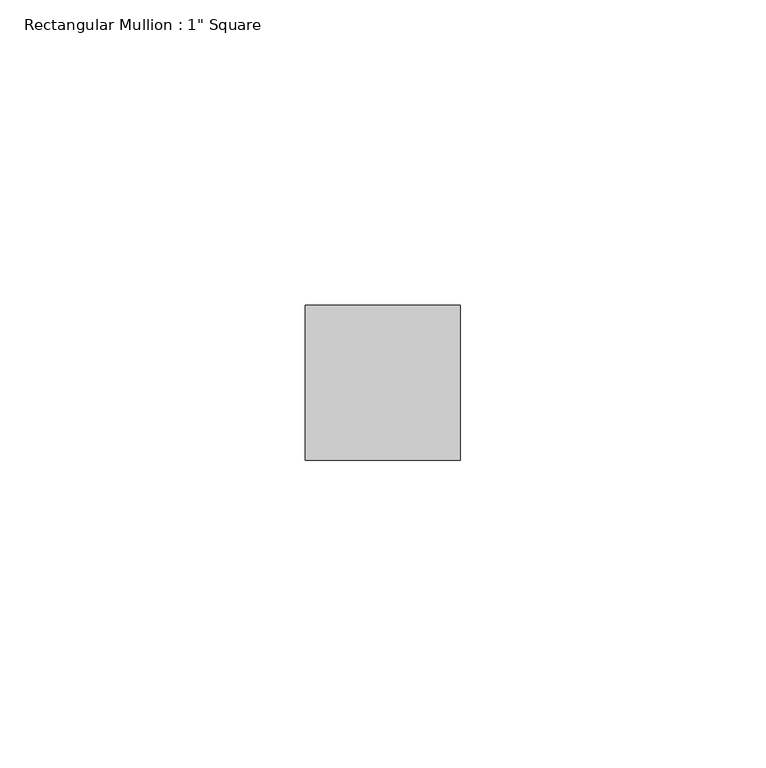
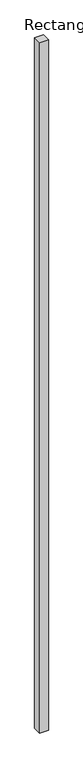
"""IFC4 building model written with IfcOpenShell, lengths in millimetres: member geometry."""

from ifc_helpers import new_model, si_unit, frame, origin, place, context, project, spatial, polyline, outline, extrude, source, transform, mapped, element, save


def member_c125f493(model_context):
    return source(origin(), model_context, "Body", "SweptSolid", [
        extrude(outline(polyline([(12.7, 12.7), (12.7, -12.7), (-12.7, -12.7), (-12.7, 12.7), (12.7, 12.7)])), frame((0.0, 0.0, -2139.95), z_axis=(0.0, 0.0, 1.0), x_axis=(1.0, 0.0, 0.0)), (0.0, 0.0, 1.0), 2139.95),
    ])


if __name__ == "__main__":
    model = new_model("IFC4")
    model_context = context("Model", 3, world=origin())
    ifc_project = project(units=[si_unit("LENGTHUNIT", "METRE", prefix="MILLI")], contexts=[model_context])
    site = spatial("IfcSite", under=ifc_project)
    building = spatial("IfcBuilding", under=site)
    placement = place(None, origin())
    member_shape = member_c125f493(model_context)
    element("IfcMember", 1, ObjectType="Rectangular Mullion : 1\" Square", at=placement, inside=building, context=model_context, shape_type="MappedRepresentation", body=[
        mapped(member_shape, transform((0.0, 0.0, 0.0), x_axis=(1.0, 0.0, 0.0), y_axis=(0.0, 1.0, 0.0), z_axis=(0.0, 0.0, 1.0))),
    ])
    save(model, "model.ifc")

# Revit data of these elements
# Type "Rectangular Mullion : 1\" Square"
#   built-in parameter 1007304 = 0.0833333 (stored number, unit not read)
#   built-in parameter 1007301 = 0.0416667 (stored number, unit not read)
#   built-in parameter 1007300 = 0.0416667 (stored number, unit not read)
# Element 1 (IfcMember, "Rectangular Mullion : 1\" Square")
#   Materials on its faces: "Aluminum"
# Materials
#   "Aluminum": class "Metal", colour RGB 247 247 247, transparency 0, Description = "Aluminum 6061", Cost = 0
